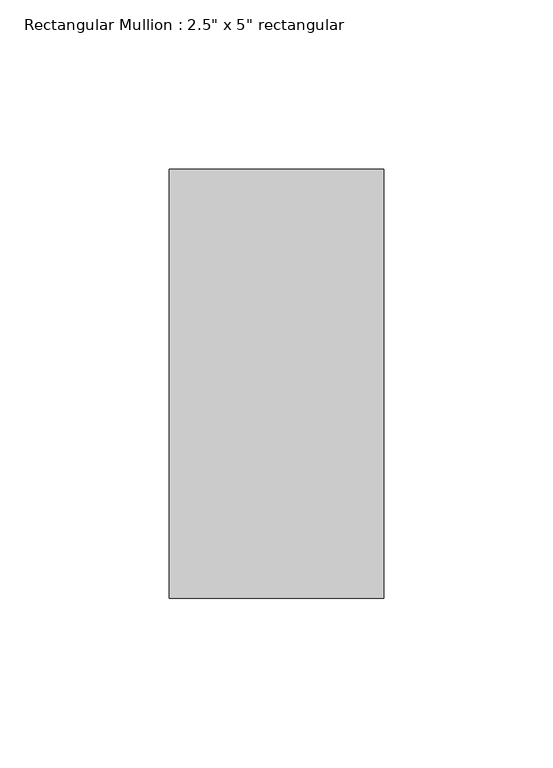
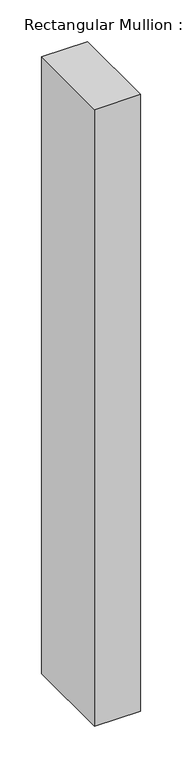
"""IFC4 building model written with IfcOpenShell, lengths in millimetres: member geometry."""

from ifc_helpers import new_model, si_unit, frame, origin, place, context, project, spatial, polyline, outline, extrude, source, transform, mapped, element, save


def member_cb167e66(model_context):
    return source(origin(), model_context, "Body", "SweptSolid", [
        extrude(outline(polyline([(31.75, 63.5), (31.75, -63.5), (-31.75, -63.5), (-31.75, 63.5), (31.75, 63.5)])), frame((0.0, 0.0, -902.5301773), z_axis=(0.0, 0.0, 1.0), x_axis=(1.0, 0.0, 0.0)), (0.0, 0.0, 1.0), 902.5301773),
    ])


if __name__ == "__main__":
    model = new_model("IFC4")
    model_context = context("Model", 3, world=origin())
    ifc_project = project(units=[si_unit("LENGTHUNIT", "METRE", prefix="MILLI")], contexts=[model_context])
    site = spatial("IfcSite", under=ifc_project)
    building = spatial("IfcBuilding", under=site)
    placement = place(None, origin())
    member_shape = member_cb167e66(model_context)
    element("IfcMember", 1, ObjectType="Rectangular Mullion : 2.5\" x 5\" rectangular", at=placement, inside=building, context=model_context, shape_type="MappedRepresentation", body=[
        mapped(member_shape, transform((0.0, 0.0, 0.0), x_axis=(1.0, 0.0, 0.0), y_axis=(0.0, 1.0, 0.0), z_axis=(0.0, 0.0, 1.0))),
    ])
    save(model, "model.ifc")

# Revit data of these elements
# Type "Rectangular Mullion : 2.5\" x 5\" rectangular"
#   built-in parameter 1007304 = 0.416667 (stored number, unit not read)
#   built-in parameter 1007301 = 0.104167 (stored number, unit not read)
#   built-in parameter 1007300 = 0.104167 (stored number, unit not read)
# Element 1 (IfcMember, "Rectangular Mullion : 2.5\" x 5\" rectangular")
#   Materials on its faces: "Aluminum"
# Materials
#   "Aluminum": class "Metal", colour RGB 247 247 247, transparency 0, Description = "Aluminum 6061", Cost = 0
